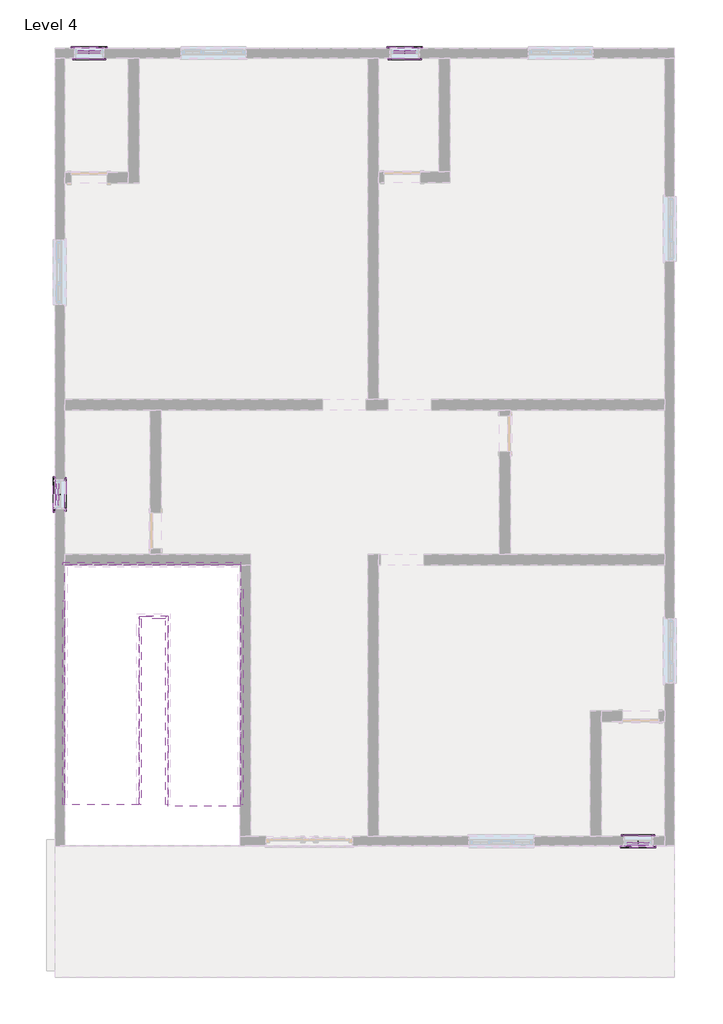
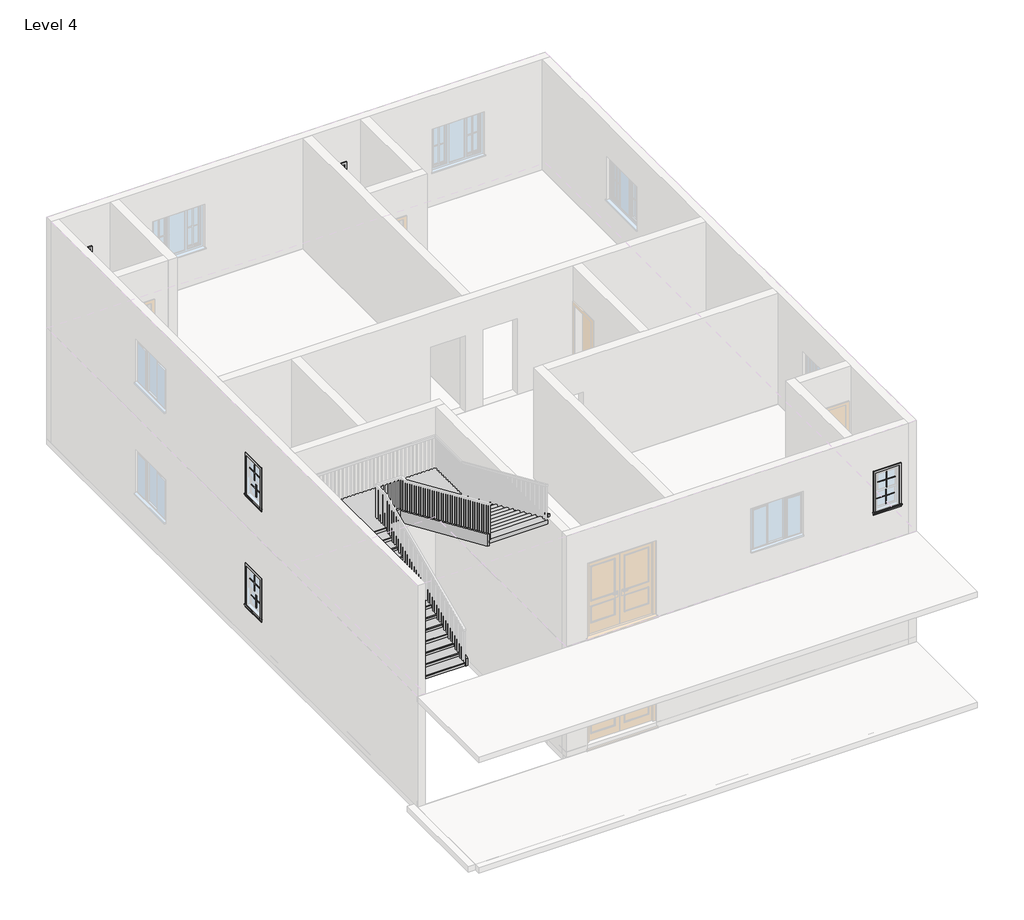
# One storey, part 5 of 5: 48 proxies, 6 members, 1 stair flight.
"""IFC4 building model written with IfcOpenShell, lengths in millimetres."""

from ifc_helpers import new_model, si_unit, frame, origin, place, context, project, spatial, polyline, outline, extrude, transform, mapped, element, save
from components import muntin_pattern_2x2_muntin_pattern_2x2_eba6c5fb, trim_window_exterior_flat_with_sill_278e6a94, trim_window_interior_flat_picture_frame_e9fd5f45, stair_flight_303fa83b

model = new_model("IFC4")

# Units and contexts
model_context = context("Model", 3, world=origin())
ifc_project = project(units=[si_unit("LENGTHUNIT", "METRE", prefix="MILLI")], contexts=[model_context])

# Site, building, storey
site = spatial("IfcSite", under=ifc_project)
building = spatial("IfcBuilding", under=site)
storey = spatial("IfcBuildingStorey", under=building, Name="Level 4", Elevation=9144.0)

# Proxies
placement = place(None, origin())
muntin_pattern_2x2_muntin_pattern_2x2_shape = muntin_pattern_2x2_muntin_pattern_2x2_eba6c5fb(model_context)
element("IfcBuildingElementProxy", 1, Name="Muntin Pattern_2x2 : Muntin Pattern_2x2", ObjectType="Muntin Pattern_2x2 : Muntin Pattern_2x2", at=placement, inside=storey, context=model_context, shape_type="MappedRepresentation", body=[
    mapped(muntin_pattern_2x2_muntin_pattern_2x2_shape, transform((-7722.7165084, -455.2217109, 10614.025), x_axis=(0.0, 1.0, 0.0), y_axis=(-1.0, 0.0, 0.0), z_axis=(0.0, 0.0, 1.0))),
])
element("IfcBuildingElementProxy", 2, Name="Muntin Pattern_2x2 : Muntin Pattern_2x2", ObjectType="Muntin Pattern_2x2 : Muntin Pattern_2x2", at=placement, inside=storey, context=model_context, shape_type="MappedRepresentation", body=[
    mapped(muntin_pattern_2x2_muntin_pattern_2x2_shape, transform((-7678.2665084, -455.2217109, 10134.6), x_axis=(0.0, 1.0, 0.0), y_axis=(-1.0, 0.0, 0.0), z_axis=(0.0, 0.0, 1.0))),
])
element("IfcBuildingElementProxy", 3, Name="Muntin Pattern_2x2 : Muntin Pattern_2x2", ObjectType="Muntin Pattern_2x2 : Muntin Pattern_2x2", at=placement, inside=storey, context=model_context, shape_type="MappedRepresentation", body=[
    mapped(muntin_pattern_2x2_muntin_pattern_2x2_shape, transform((-7046.4415084, 8872.5685985, 10614.025), x_axis=(1.0, 0.0, 0.0), y_axis=(0.0, 1.0, 0.0), z_axis=(0.0, 0.0, 1.0))),
])
element("IfcBuildingElementProxy", 4, Name="Muntin Pattern_2x2 : Muntin Pattern_2x2", ObjectType="Muntin Pattern_2x2 : Muntin Pattern_2x2", at=placement, inside=storey, context=model_context, shape_type="MappedRepresentation", body=[
    mapped(muntin_pattern_2x2_muntin_pattern_2x2_shape, transform((-7046.4415084, 8828.1185985, 10134.6), x_axis=(1.0, 0.0, 0.0), y_axis=(0.0, 1.0, 0.0), z_axis=(0.0, 0.0, 1.0))),
])
element("IfcBuildingElementProxy", 5, Name="Muntin Pattern_2x2 : Muntin Pattern_2x2", ObjectType="Muntin Pattern_2x2 : Muntin Pattern_2x2", at=placement, inside=storey, context=model_context, shape_type="MappedRepresentation", body=[
    mapped(muntin_pattern_2x2_muntin_pattern_2x2_shape, transform((-417.0415084, 8872.5685985, 10614.025), x_axis=(1.0, 0.0, 0.0), y_axis=(0.0, 1.0, 0.0), z_axis=(0.0, 0.0, 1.0))),
])
element("IfcBuildingElementProxy", 6, Name="Muntin Pattern_2x2 : Muntin Pattern_2x2", ObjectType="Muntin Pattern_2x2 : Muntin Pattern_2x2", at=placement, inside=storey, context=model_context, shape_type="MappedRepresentation", body=[
    mapped(muntin_pattern_2x2_muntin_pattern_2x2_shape, transform((-417.0415084, 8828.1185985, 10134.6), x_axis=(1.0, 0.0, 0.0), y_axis=(0.0, 1.0, 0.0), z_axis=(0.0, 0.0, 1.0))),
])
element("IfcBuildingElementProxy", 7, Name="Muntin Pattern_2x2 : Muntin Pattern_2x2", ObjectType="Muntin Pattern_2x2 : Muntin Pattern_2x2", at=placement, inside=storey, context=model_context, shape_type="MappedRepresentation", body=[
    mapped(muntin_pattern_2x2_muntin_pattern_2x2_shape, transform((4485.1584916, -7796.1814015, 10614.025), x_axis=(-1.0, 0.0, 0.0), y_axis=(0.0, -1.0, 0.0), z_axis=(0.0, 0.0, 1.0))),
])
element("IfcBuildingElementProxy", 8, Name="Muntin Pattern_2x2 : Muntin Pattern_2x2", ObjectType="Muntin Pattern_2x2 : Muntin Pattern_2x2", at=placement, inside=storey, context=model_context, shape_type="MappedRepresentation", body=[
    mapped(muntin_pattern_2x2_muntin_pattern_2x2_shape, transform((4485.1584916, -7751.7314015, 10134.6), x_axis=(-1.0, 0.0, 0.0), y_axis=(0.0, -1.0, 0.0), z_axis=(0.0, 0.0, 1.0))),
])
element("IfcBuildingElementProxy", 9, Name="Muntin Pattern_2x2 : Muntin Pattern_2x2", ObjectType="Muntin Pattern_2x2 : Muntin Pattern_2x2", at=placement, inside=storey, context=model_context, shape_type="MappedRepresentation", body=[
    mapped(muntin_pattern_2x2_muntin_pattern_2x2_shape, transform((-7722.7165084, -455.2217109, 10614.025), x_axis=(0.0, 1.0, 0.0), y_axis=(-1.0, 0.0, 0.0), z_axis=(0.0, 0.0, 1.0))),
])
element("IfcBuildingElementProxy", 10, Name="Muntin Pattern_2x2 : Muntin Pattern_2x2", ObjectType="Muntin Pattern_2x2 : Muntin Pattern_2x2", at=placement, inside=storey, context=model_context, shape_type="MappedRepresentation", body=[
    mapped(muntin_pattern_2x2_muntin_pattern_2x2_shape, transform((-7678.2665084, -455.2217109, 10134.6), x_axis=(0.0, 1.0, 0.0), y_axis=(-1.0, 0.0, 0.0), z_axis=(0.0, 0.0, 1.0))),
])
element("IfcBuildingElementProxy", 11, Name="Muntin Pattern_2x2 : Muntin Pattern_2x2", ObjectType="Muntin Pattern_2x2 : Muntin Pattern_2x2", at=placement, inside=storey, context=model_context, shape_type="MappedRepresentation", body=[
    mapped(muntin_pattern_2x2_muntin_pattern_2x2_shape, transform((-7046.4415084, 8872.5685985, 10614.025), x_axis=(1.0, 0.0, 0.0), y_axis=(0.0, 1.0, 0.0), z_axis=(0.0, 0.0, 1.0))),
])
element("IfcBuildingElementProxy", 12, Name="Muntin Pattern_2x2 : Muntin Pattern_2x2", ObjectType="Muntin Pattern_2x2 : Muntin Pattern_2x2", at=placement, inside=storey, context=model_context, shape_type="MappedRepresentation", body=[
    mapped(muntin_pattern_2x2_muntin_pattern_2x2_shape, transform((-7046.4415084, 8828.1185985, 10134.6), x_axis=(1.0, 0.0, 0.0), y_axis=(0.0, 1.0, 0.0), z_axis=(0.0, 0.0, 1.0))),
])
element("IfcBuildingElementProxy", 13, Name="Muntin Pattern_2x2 : Muntin Pattern_2x2", ObjectType="Muntin Pattern_2x2 : Muntin Pattern_2x2", at=placement, inside=storey, context=model_context, shape_type="MappedRepresentation", body=[
    mapped(muntin_pattern_2x2_muntin_pattern_2x2_shape, transform((-417.0415084, 8872.5685985, 10614.025), x_axis=(1.0, 0.0, 0.0), y_axis=(0.0, 1.0, 0.0), z_axis=(0.0, 0.0, 1.0))),
])
element("IfcBuildingElementProxy", 14, Name="Muntin Pattern_2x2 : Muntin Pattern_2x2", ObjectType="Muntin Pattern_2x2 : Muntin Pattern_2x2", at=placement, inside=storey, context=model_context, shape_type="MappedRepresentation", body=[
    mapped(muntin_pattern_2x2_muntin_pattern_2x2_shape, transform((-417.0415084, 8828.1185985, 10134.6), x_axis=(1.0, 0.0, 0.0), y_axis=(0.0, 1.0, 0.0), z_axis=(0.0, 0.0, 1.0))),
])
element("IfcBuildingElementProxy", 15, Name="Muntin Pattern_2x2 : Muntin Pattern_2x2", ObjectType="Muntin Pattern_2x2 : Muntin Pattern_2x2", at=placement, inside=storey, context=model_context, shape_type="MappedRepresentation", body=[
    mapped(muntin_pattern_2x2_muntin_pattern_2x2_shape, transform((4485.1584916, -7796.1814015, 10614.025), x_axis=(-1.0, 0.0, 0.0), y_axis=(0.0, -1.0, 0.0), z_axis=(0.0, 0.0, 1.0))),
])
element("IfcBuildingElementProxy", 16, Name="Muntin Pattern_2x2 : Muntin Pattern_2x2", ObjectType="Muntin Pattern_2x2 : Muntin Pattern_2x2", at=placement, inside=storey, context=model_context, shape_type="MappedRepresentation", body=[
    mapped(muntin_pattern_2x2_muntin_pattern_2x2_shape, transform((4485.1584916, -7751.7314015, 10134.6), x_axis=(-1.0, 0.0, 0.0), y_axis=(0.0, -1.0, 0.0), z_axis=(0.0, 0.0, 1.0))),
])
element("IfcBuildingElementProxy", 17, Name="Muntin Pattern_2x2 : Muntin Pattern_2x2", ObjectType="Muntin Pattern_2x2 : Muntin Pattern_2x2", at=placement, inside=storey, context=model_context, shape_type="MappedRepresentation", body=[
    mapped(muntin_pattern_2x2_muntin_pattern_2x2_shape, transform((-7722.7165084, -455.2217109, 13662.025), x_axis=(0.0, 1.0, 0.0), y_axis=(-1.0, 0.0, 0.0), z_axis=(0.0, 0.0, 1.0))),
])
element("IfcBuildingElementProxy", 18, Name="Muntin Pattern_2x2 : Muntin Pattern_2x2", ObjectType="Muntin Pattern_2x2 : Muntin Pattern_2x2", at=placement, inside=storey, context=model_context, shape_type="MappedRepresentation", body=[
    mapped(muntin_pattern_2x2_muntin_pattern_2x2_shape, transform((-7678.2665084, -455.2217109, 13182.6), x_axis=(0.0, 1.0, 0.0), y_axis=(-1.0, 0.0, 0.0), z_axis=(0.0, 0.0, 1.0))),
])
element("IfcBuildingElementProxy", 19, Name="Muntin Pattern_2x2 : Muntin Pattern_2x2", ObjectType="Muntin Pattern_2x2 : Muntin Pattern_2x2", at=placement, inside=storey, context=model_context, shape_type="MappedRepresentation", body=[
    mapped(muntin_pattern_2x2_muntin_pattern_2x2_shape, transform((-7046.4415084, 8872.5685985, 13662.025), x_axis=(1.0, 0.0, 0.0), y_axis=(0.0, 1.0, 0.0), z_axis=(0.0, 0.0, 1.0))),
])
element("IfcBuildingElementProxy", 20, Name="Muntin Pattern_2x2 : Muntin Pattern_2x2", ObjectType="Muntin Pattern_2x2 : Muntin Pattern_2x2", at=placement, inside=storey, context=model_context, shape_type="MappedRepresentation", body=[
    mapped(muntin_pattern_2x2_muntin_pattern_2x2_shape, transform((-7046.4415084, 8828.1185985, 13182.6), x_axis=(1.0, 0.0, 0.0), y_axis=(0.0, 1.0, 0.0), z_axis=(0.0, 0.0, 1.0))),
])
element("IfcBuildingElementProxy", 21, Name="Muntin Pattern_2x2 : Muntin Pattern_2x2", ObjectType="Muntin Pattern_2x2 : Muntin Pattern_2x2", at=placement, inside=storey, context=model_context, shape_type="MappedRepresentation", body=[
    mapped(muntin_pattern_2x2_muntin_pattern_2x2_shape, transform((-417.0415084, 8872.5685985, 13662.025), x_axis=(1.0, 0.0, 0.0), y_axis=(0.0, 1.0, 0.0), z_axis=(0.0, 0.0, 1.0))),
])
element("IfcBuildingElementProxy", 22, Name="Muntin Pattern_2x2 : Muntin Pattern_2x2", ObjectType="Muntin Pattern_2x2 : Muntin Pattern_2x2", at=placement, inside=storey, context=model_context, shape_type="MappedRepresentation", body=[
    mapped(muntin_pattern_2x2_muntin_pattern_2x2_shape, transform((-417.0415084, 8828.1185985, 13182.6), x_axis=(1.0, 0.0, 0.0), y_axis=(0.0, 1.0, 0.0), z_axis=(0.0, 0.0, 1.0))),
])
element("IfcBuildingElementProxy", 23, Name="Muntin Pattern_2x2 : Muntin Pattern_2x2", ObjectType="Muntin Pattern_2x2 : Muntin Pattern_2x2", at=placement, inside=storey, context=model_context, shape_type="MappedRepresentation", body=[
    mapped(muntin_pattern_2x2_muntin_pattern_2x2_shape, transform((4485.1584916, -7796.1814015, 13662.025), x_axis=(-1.0, 0.0, 0.0), y_axis=(0.0, -1.0, 0.0), z_axis=(0.0, 0.0, 1.0))),
])
element("IfcBuildingElementProxy", 24, Name="Muntin Pattern_2x2 : Muntin Pattern_2x2", ObjectType="Muntin Pattern_2x2 : Muntin Pattern_2x2", at=placement, inside=storey, context=model_context, shape_type="MappedRepresentation", body=[
    mapped(muntin_pattern_2x2_muntin_pattern_2x2_shape, transform((4485.1584916, -7751.7314015, 13182.6), x_axis=(-1.0, 0.0, 0.0), y_axis=(0.0, -1.0, 0.0), z_axis=(0.0, 0.0, 1.0))),
])
trim_window_exterior_flat_with_sill_shape = trim_window_exterior_flat_with_sill_278e6a94(model_context)
element("IfcBuildingElementProxy", 25, Name="Trim-Window-Exterior-Flat : with Sill", ObjectType="Trim-Window-Exterior-Flat : with Sill", at=placement, inside=storey, context=model_context, shape_type="MappedRepresentation", body=[
    mapped(trim_window_exterior_flat_with_sill_shape, transform((-7757.6415084, -455.2217109, 11125.2), x_axis=(0.0, -1.0, 0.0), y_axis=(0.0, 0.0, 1.0), z_axis=(-1.0, 0.0, 0.0))),
])
element("IfcBuildingElementProxy", 26, Name="Trim-Window-Exterior-Flat : with Sill", ObjectType="Trim-Window-Exterior-Flat : with Sill", at=placement, inside=storey, context=model_context, shape_type="MappedRepresentation", body=[
    mapped(trim_window_exterior_flat_with_sill_shape, transform((-7046.4415084, 8907.4935985, 11125.2), x_axis=(-1.0, 0.0, 0.0), y_axis=(0.0, 0.0, 1.0), z_axis=(0.0, 1.0, 0.0))),
])
element("IfcBuildingElementProxy", 27, Name="Trim-Window-Exterior-Flat : with Sill", ObjectType="Trim-Window-Exterior-Flat : with Sill", at=placement, inside=storey, context=model_context, shape_type="MappedRepresentation", body=[
    mapped(trim_window_exterior_flat_with_sill_shape, transform((-417.0415084, 8907.4935985, 11125.2), x_axis=(-1.0, 0.0, 0.0), y_axis=(0.0, 0.0, 1.0), z_axis=(0.0, 1.0, 0.0))),
])
element("IfcBuildingElementProxy", 28, Name="Trim-Window-Exterior-Flat : with Sill", ObjectType="Trim-Window-Exterior-Flat : with Sill", at=placement, inside=storey, context=model_context, shape_type="MappedRepresentation", body=[
    mapped(trim_window_exterior_flat_with_sill_shape, transform((4485.1584916, -7831.1064015, 11125.2), x_axis=(1.0, 0.0, 0.0), y_axis=(0.0, 0.0, 1.0), z_axis=(0.0, -1.0, 0.0))),
])
element("IfcBuildingElementProxy", 29, Name="Trim-Window-Exterior-Flat : with Sill", ObjectType="Trim-Window-Exterior-Flat : with Sill", at=placement, inside=storey, context=model_context, shape_type="MappedRepresentation", body=[
    mapped(trim_window_exterior_flat_with_sill_shape, transform((-7757.6415084, -455.2217109, 11125.2), x_axis=(0.0, -1.0, 0.0), y_axis=(0.0, 0.0, 1.0), z_axis=(-1.0, 0.0, 0.0))),
])
element("IfcBuildingElementProxy", 30, Name="Trim-Window-Exterior-Flat : with Sill", ObjectType="Trim-Window-Exterior-Flat : with Sill", at=placement, inside=storey, context=model_context, shape_type="MappedRepresentation", body=[
    mapped(trim_window_exterior_flat_with_sill_shape, transform((-7046.4415084, 8907.4935985, 11125.2), x_axis=(-1.0, 0.0, 0.0), y_axis=(0.0, 0.0, 1.0), z_axis=(0.0, 1.0, 0.0))),
])
element("IfcBuildingElementProxy", 31, Name="Trim-Window-Exterior-Flat : with Sill", ObjectType="Trim-Window-Exterior-Flat : with Sill", at=placement, inside=storey, context=model_context, shape_type="MappedRepresentation", body=[
    mapped(trim_window_exterior_flat_with_sill_shape, transform((-417.0415084, 8907.4935985, 11125.2), x_axis=(-1.0, 0.0, 0.0), y_axis=(0.0, 0.0, 1.0), z_axis=(0.0, 1.0, 0.0))),
])
element("IfcBuildingElementProxy", 32, Name="Trim-Window-Exterior-Flat : with Sill", ObjectType="Trim-Window-Exterior-Flat : with Sill", at=placement, inside=storey, context=model_context, shape_type="MappedRepresentation", body=[
    mapped(trim_window_exterior_flat_with_sill_shape, transform((4485.1584916, -7831.1064015, 11125.2), x_axis=(1.0, 0.0, 0.0), y_axis=(0.0, 0.0, 1.0), z_axis=(0.0, -1.0, 0.0))),
])
element("IfcBuildingElementProxy", 33, Name="Trim-Window-Exterior-Flat : with Sill", ObjectType="Trim-Window-Exterior-Flat : with Sill", at=placement, inside=storey, context=model_context, shape_type="MappedRepresentation", body=[
    mapped(trim_window_exterior_flat_with_sill_shape, transform((-7757.6415084, -455.2217109, 14173.2), x_axis=(0.0, -1.0, 0.0), y_axis=(0.0, 0.0, 1.0), z_axis=(-1.0, 0.0, 0.0))),
])
element("IfcBuildingElementProxy", 34, Name="Trim-Window-Exterior-Flat : with Sill", ObjectType="Trim-Window-Exterior-Flat : with Sill", at=placement, inside=storey, context=model_context, shape_type="MappedRepresentation", body=[
    mapped(trim_window_exterior_flat_with_sill_shape, transform((-7046.4415084, 8907.4935985, 14173.2), x_axis=(-1.0, 0.0, 0.0), y_axis=(0.0, 0.0, 1.0), z_axis=(0.0, 1.0, 0.0))),
])
element("IfcBuildingElementProxy", 35, Name="Trim-Window-Exterior-Flat : with Sill", ObjectType="Trim-Window-Exterior-Flat : with Sill", at=placement, inside=storey, context=model_context, shape_type="MappedRepresentation", body=[
    mapped(trim_window_exterior_flat_with_sill_shape, transform((-417.0415084, 8907.4935985, 14173.2), x_axis=(-1.0, 0.0, 0.0), y_axis=(0.0, 0.0, 1.0), z_axis=(0.0, 1.0, 0.0))),
])
element("IfcBuildingElementProxy", 36, Name="Trim-Window-Exterior-Flat : with Sill", ObjectType="Trim-Window-Exterior-Flat : with Sill", at=placement, inside=storey, context=model_context, shape_type="MappedRepresentation", body=[
    mapped(trim_window_exterior_flat_with_sill_shape, transform((4485.1584916, -7831.1064015, 14173.2), x_axis=(1.0, 0.0, 0.0), y_axis=(0.0, 0.0, 1.0), z_axis=(0.0, -1.0, 0.0))),
])
trim_window_interior_flat_picture_frame_shape = trim_window_interior_flat_picture_frame_e9fd5f45(model_context)
element("IfcBuildingElementProxy", 37, Name="Trim-Window-Interior-Flat : Picture Frame", ObjectType="Trim-Window-Interior-Flat : Picture Frame", at=placement, inside=storey, context=model_context, shape_type="MappedRepresentation", body=[
    mapped(trim_window_interior_flat_picture_frame_shape, transform((-7554.4415084, -455.2217109, 11125.2), x_axis=(0.0, 1.0, 0.0), y_axis=(0.0, 0.0, 1.0), z_axis=(1.0, 0.0, 0.0))),
])
element("IfcBuildingElementProxy", 38, Name="Trim-Window-Interior-Flat : Picture Frame", ObjectType="Trim-Window-Interior-Flat : Picture Frame", at=placement, inside=storey, context=model_context, shape_type="MappedRepresentation", body=[
    mapped(trim_window_interior_flat_picture_frame_shape, transform((-7046.4415084, 8704.2935985, 11125.2), x_axis=(1.0, 0.0, 0.0), y_axis=(0.0, 0.0, 1.0), z_axis=(0.0, -1.0, 0.0))),
])
element("IfcBuildingElementProxy", 39, Name="Trim-Window-Interior-Flat : Picture Frame", ObjectType="Trim-Window-Interior-Flat : Picture Frame", at=placement, inside=storey, context=model_context, shape_type="MappedRepresentation", body=[
    mapped(trim_window_interior_flat_picture_frame_shape, transform((-417.0415084, 8704.2935985, 11125.2), x_axis=(1.0, 0.0, 0.0), y_axis=(0.0, 0.0, 1.0), z_axis=(0.0, -1.0, 0.0))),
])
element("IfcBuildingElementProxy", 40, Name="Trim-Window-Interior-Flat : Picture Frame", ObjectType="Trim-Window-Interior-Flat : Picture Frame", at=placement, inside=storey, context=model_context, shape_type="MappedRepresentation", body=[
    mapped(trim_window_interior_flat_picture_frame_shape, transform((4485.1584916, -7627.9064015, 11125.2), x_axis=(-1.0, 0.0, 0.0), y_axis=(0.0, 0.0, 1.0), z_axis=(0.0, 1.0, 0.0))),
])
element("IfcBuildingElementProxy", 41, Name="Trim-Window-Interior-Flat : Picture Frame", ObjectType="Trim-Window-Interior-Flat : Picture Frame", at=placement, inside=storey, context=model_context, shape_type="MappedRepresentation", body=[
    mapped(trim_window_interior_flat_picture_frame_shape, transform((-7554.4415084, -455.2217109, 11125.2), x_axis=(0.0, 1.0, 0.0), y_axis=(0.0, 0.0, 1.0), z_axis=(1.0, 0.0, 0.0))),
])
element("IfcBuildingElementProxy", 42, Name="Trim-Window-Interior-Flat : Picture Frame", ObjectType="Trim-Window-Interior-Flat : Picture Frame", at=placement, inside=storey, context=model_context, shape_type="MappedRepresentation", body=[
    mapped(trim_window_interior_flat_picture_frame_shape, transform((-7046.4415084, 8704.2935985, 11125.2), x_axis=(1.0, 0.0, 0.0), y_axis=(0.0, 0.0, 1.0), z_axis=(0.0, -1.0, 0.0))),
])
element("IfcBuildingElementProxy", 43, Name="Trim-Window-Interior-Flat : Picture Frame", ObjectType="Trim-Window-Interior-Flat : Picture Frame", at=placement, inside=storey, context=model_context, shape_type="MappedRepresentation", body=[
    mapped(trim_window_interior_flat_picture_frame_shape, transform((-417.0415084, 8704.2935985, 11125.2), x_axis=(1.0, 0.0, 0.0), y_axis=(0.0, 0.0, 1.0), z_axis=(0.0, -1.0, 0.0))),
])
element("IfcBuildingElementProxy", 44, Name="Trim-Window-Interior-Flat : Picture Frame", ObjectType="Trim-Window-Interior-Flat : Picture Frame", at=placement, inside=storey, context=model_context, shape_type="MappedRepresentation", body=[
    mapped(trim_window_interior_flat_picture_frame_shape, transform((4485.1584916, -7627.9064015, 11125.2), x_axis=(-1.0, 0.0, 0.0), y_axis=(0.0, 0.0, 1.0), z_axis=(0.0, 1.0, 0.0))),
])
element("IfcBuildingElementProxy", 45, Name="Trim-Window-Interior-Flat : Picture Frame", ObjectType="Trim-Window-Interior-Flat : Picture Frame", at=placement, inside=storey, context=model_context, shape_type="MappedRepresentation", body=[
    mapped(trim_window_interior_flat_picture_frame_shape, transform((-7554.4415084, -455.2217109, 14173.2), x_axis=(0.0, 1.0, 0.0), y_axis=(0.0, 0.0, 1.0), z_axis=(1.0, 0.0, 0.0))),
])
element("IfcBuildingElementProxy", 46, Name="Trim-Window-Interior-Flat : Picture Frame", ObjectType="Trim-Window-Interior-Flat : Picture Frame", at=placement, inside=storey, context=model_context, shape_type="MappedRepresentation", body=[
    mapped(trim_window_interior_flat_picture_frame_shape, transform((-7046.4415084, 8704.2935985, 14173.2), x_axis=(1.0, 0.0, 0.0), y_axis=(0.0, 0.0, 1.0), z_axis=(0.0, -1.0, 0.0))),
])
element("IfcBuildingElementProxy", 47, Name="Trim-Window-Interior-Flat : Picture Frame", ObjectType="Trim-Window-Interior-Flat : Picture Frame", at=placement, inside=storey, context=model_context, shape_type="MappedRepresentation", body=[
    mapped(trim_window_interior_flat_picture_frame_shape, transform((-417.0415084, 8704.2935985, 14173.2), x_axis=(1.0, 0.0, 0.0), y_axis=(0.0, 0.0, 1.0), z_axis=(0.0, -1.0, 0.0))),
])
element("IfcBuildingElementProxy", 48, Name="Trim-Window-Interior-Flat : Picture Frame", ObjectType="Trim-Window-Interior-Flat : Picture Frame", at=placement, inside=storey, context=model_context, shape_type="MappedRepresentation", body=[
    mapped(trim_window_interior_flat_picture_frame_shape, transform((4485.1584916, -7627.9064015, 14173.2), x_axis=(-1.0, 0.0, 0.0), y_axis=(0.0, 0.0, 1.0), z_axis=(0.0, 1.0, 0.0))),
])

# Members
element("IfcMember", 49, ObjectType="Stringer - 2\" Width", at=placement, inside=storey, context=model_context, shape_type="SweptSolid", body=[
    extrude(outline(polyline([(-6973.0610642, 11887.2), (-6973.0610642, 12086.0550815), (-3441.822613, 13639.8), (-2685.0041973, 13639.8), (-6668.1860155, 11887.2), (-6973.0610642, 11887.2)])), frame((-7605.2415084, 0.0, 0.0), z_axis=(1.0, 0.0, 0.0), x_axis=(0.0, 1.0, 0.0)), (0.0, 0.0, 1.0), 50.8),
])
element("IfcMember", 50, ObjectType="Stringer - 2\" Width", at=placement, inside=storey, context=model_context, shape_type="SweptSolid", body=[
    extrude(outline(polyline([(-7605.2415084, -1928.4217109), (-7605.2415084, -1877.6217109), (-3866.3290366, -1877.6217109), (-3866.3290366, -1928.4217109), (-7605.2415084, -1928.4217109)])), frame((0.0, 0.0, 13335.0), z_axis=(0.0, 0.0, 1.0), x_axis=(1.0, 0.0, 0.0)), (0.0, 0.0, 1.0), 304.8),
])
element("IfcMember", 51, ObjectType="Stringer - 2\" Width", at=placement, inside=storey, context=model_context, shape_type="SweptSolid", body=[
    extrude(outline(polyline([(-3202.3906584, 13335.0), (-6973.0610642, 14994.0949786), (-6973.0610642, 15327.0950815), (-2445.5722427, 13335.0), (-3202.3906584, 13335.0)])), frame((-3866.3290366, 0.0, 0.0), z_axis=(1.0, 0.0, 0.0), x_axis=(0.0, 1.0, 0.0)), (0.0, 0.0, 1.0), 50.8),
])
element("IfcMember", 52, ObjectType="Stringer - 2\" Width", at=placement, inside=storey, context=model_context, shape_type="SweptSolid", body=[
    extrude(outline(polyline([(-6973.0610642, 11887.2), (-6973.0610642, 12086.0550815), (-3441.822613, 13639.8), (-3061.4610642, 13639.8), (-3061.4610642, 13474.1589786), (-6668.1860155, 11887.2), (-6973.0610642, 11887.2)])), frame((-5999.9290366, 0.0, 0.0), z_axis=(1.0, 0.0, 0.0), x_axis=(0.0, 1.0, 0.0)), (0.0, 0.0, 1.0), 50.8),
])
element("IfcMember", 53, ObjectType="Stringer - 2\" Width", at=placement, inside=storey, context=model_context, shape_type="SweptSolid", body=[
    extrude(outline(polyline([(-5999.9290366, -3061.4610642), (-5999.9290366, -3010.6610642), (-5441.1290366, -3010.6610642), (-5441.1290366, -3061.4610642), (-5999.9290366, -3061.4610642)])), frame((0.0, 0.0, 13335.0), z_axis=(0.0, 0.0, 1.0), x_axis=(1.0, 0.0, 0.0)), (0.0, 0.0, 1.0), 304.8),
])
element("IfcMember", 54, ObjectType="Stringer - 2\" Width", at=placement, inside=storey, context=model_context, shape_type="SweptSolid", body=[
    extrude(outline(polyline([(-3010.6610642, 13583.6390815), (-3010.6610642, 13335.0), (-3202.3906584, 13335.0), (-6973.0610642, 14994.0949786), (-6973.0610642, 15327.0950815), (-3010.6610642, 13583.6390815)])), frame((-5441.1290366, 0.0, 0.0), z_axis=(1.0, 0.0, 0.0), x_axis=(0.0, 1.0, 0.0)), (0.0, 0.0, 1.0), 50.8),
])

# Stair flight
stair_flight_shape = stair_flight_303fa83b(model_context)
element("IfcStairFlight", 55, ObjectType="2\" Tread 1\" Nosing 1/4\" Riser", at=placement, inside=storey, context=model_context, shape_type="MappedRepresentation", body=[
    mapped(stair_flight_shape, transform((0.0, 0.0, 0.0), x_axis=(1.0, 0.0, 0.0), y_axis=(0.0, 1.0, 0.0), z_axis=(0.0, 0.0, 1.0))),
])

save(model, "model.ifc")

# Revit data of these elements
# Type "Muntin Pattern_2x2 : Muntin Pattern_2x2"
#   Width [instance default] = 4' - 0"
#   Thickness = 0' - 0 1/2"
#   Height [instance default] = 4' - 0"
#   Distance = 0' - 0 3/4"
#   Interior Material [instance default] = none
#   Exterior Material [instance default] = none
#   Default Elevation = 0
# Type "Trim-Window-Exterior-Flat : with Sill"
#   Trim Width = 0' - 2 1/4"
#   Trim Thickness_Picture Frame = 0' - 1 1/4"
#   Trim Thickness_with Sill = 0' - 0 3/4"
#   Sill Thickness = 0' - 1 1/4"
#   Opening Width [instance default] = 2' - 0"
#   Opening Height [instance default] = 3' - 0"
#   Default Elevation = 4' - 0"
#   Sill = yes
#   Picture Frame = no
#   Trim Material [instance default] = none
# Type "Trim-Window-Interior-Flat : Picture Frame"
#   Trim Thickness_Picture Frame = 0' - 1 1/4"
#   Trim Width = 0' - 2 1/4"
#   Trim Thickness_with Sill = 0' - 0 3/4"
#   Sill Thickness = 0' - 1 1/4"
#   Opening Width [instance default] = 2' - 0"
#   Opening Height [instance default] = 3' - 0"
#   Default Elevation = 4' - 0"
#   Sill = no
#   Picture Frame = yes
#   Trim Material [instance default] = none
# Elements 1, 2, 3, 4, 5, 6, 7, 8, 9, 10, 11, 12, 13, 14, 15, 16, 17, 18, 19, 20, 21, 22, 23, 24 (IfcBuildingElementProxy, "Muntin Pattern_2x2 : Muntin Pattern_2x2")
#   Width = 1' - 6"
#   Height = 1' - 5 1/8"
#   Interior Material = Wood - Stained
#   Exterior Material = Clad - White
#   Phase Created = New Construction
#   Materials on its faces: "Clad - White", "Wood - Stained"
# Elements 25, 26, 27, 28, 29, 30, 31, 32, 33, 34, 35, 36 (IfcBuildingElementProxy, "Trim-Window-Exterior-Flat : with Sill")
#   Opening Width = 2' - 0"
#   Opening Height = 3' - 6"
#   Trim Material = Clad - White
#   Phase Created = New Construction
#   Materials on its faces: "Clad - White"
# Elements 37, 38, 39, 40, 41, 42, 43, 44, 45, 46, 47, 48 (IfcBuildingElementProxy, "Trim-Window-Interior-Flat : Picture Frame")
#   Opening Width = 2' - 0"
#   Opening Height = 3' - 6"
#   Trim Material = Wood - Stained
#   Phase Created = New Construction
#   Materials on its faces: "Wood - Stained"
# Elements 49, 50, 51, 52, 53 (IfcMember, "Stringer - 2\" Width")
#   Phase Created = New Construction
# Element 54 (IfcMember, "Stringer - 2\" Width")
#   Phase Created = New Construction
#   Materials on its faces: "Concrete, Precast"
# Element 55 (IfcStairFlight, "2\" Tread 1\" Nosing 1/4\" Riser")
#   Phase Created = New Construction
# Materials
#   "Clad - White": class "Wood", colour RGB 242 242 238, transparency 0, Cost = 0
#   "Wood - Stained": class "Wood", colour RGB 224 178 126, transparency 0, Cost = 0
#   "Concrete, Precast": class "Concrete", colour RGB 198 187 187, transparency 0, Description = "Precast concrete", Cost = 0
